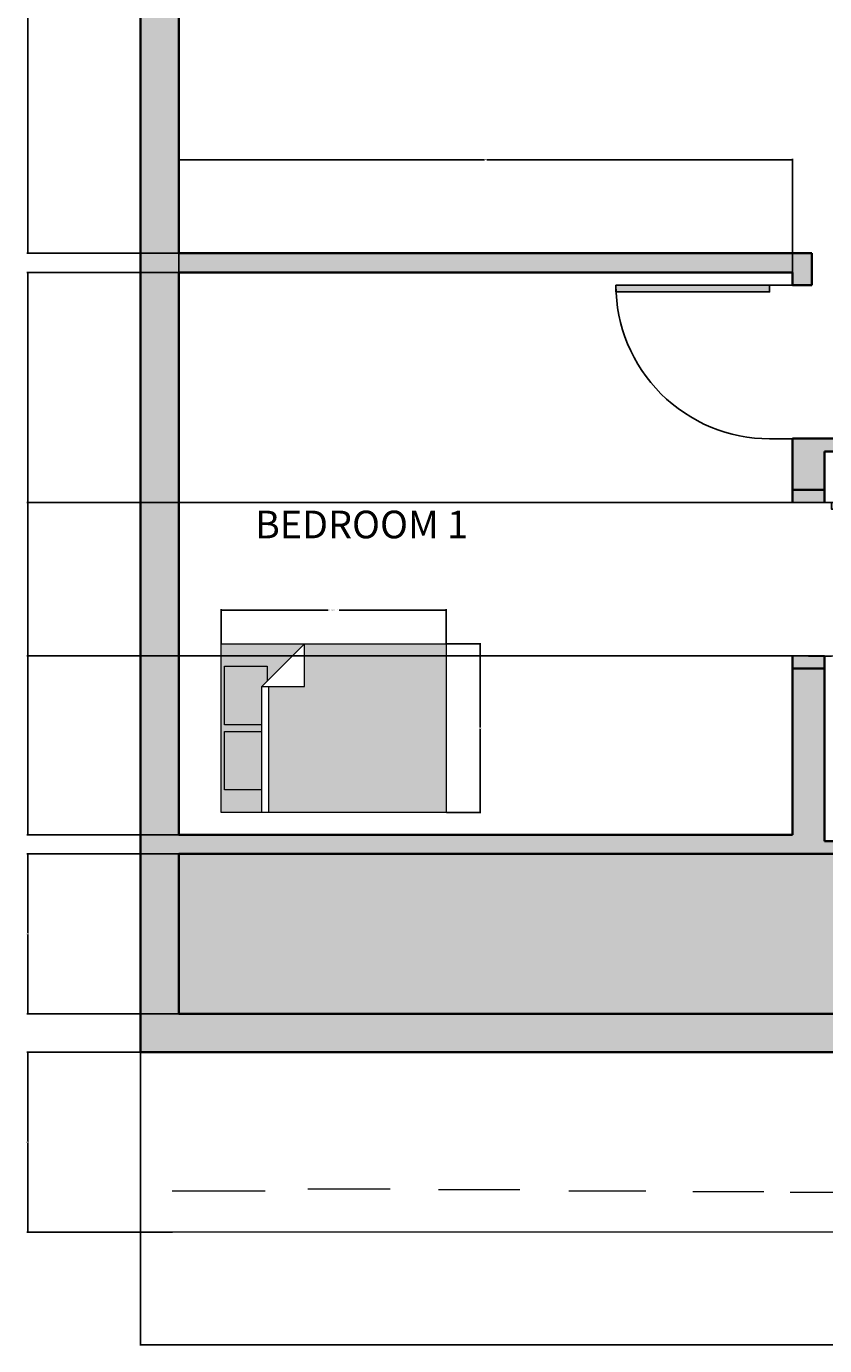
# Model space of a CAD drawing. Units: inches. Extents: x 1034 to 1730, y 674 to 1249.
# Tile 1 of 4: x 1316 to 1503, y 674 to 983. Entities that reach past the tile are written whole.
import ezdxf

# ---------------------------------------------------------------- set-up
doc = ezdxf.new("R2010")
doc.units = ezdxf.units.IN
for name, color, linetype, lineweight in [('A-ANNO-DIMS', 2, 'Continuous', 18), ('A-AREA-IDEN', 7, 'Continuous', 18), ('A-DOOR', 4, 'Continuous', 25), ('A-FURN', 9, 'Continuous', 18), ('A-FURN-PATT', 7, 'Continuous', 13), ('A-WALL', 7, 'Continuous', 35), ('A-WALL-PATT', 8, 'Continuous', 13), ('C-ROAD', 7, 'Continuous', 18)]:
    doc.layers.add(name, color=color, linetype=linetype, lineweight=lineweight)
doc.layers.add('A-DOOR-PATT', color=17, linetype='Continuous', lineweight=13, true_color=0x7b4636)
doc.layers.add('C-SITE-PATT', color=18, linetype='Continuous', lineweight=13, true_color=0x000000)
doc.styles.get("Standard").update_dxf_attribs({"font": 'arial.ttf'})
doc.dimstyles.get("Standard").update_dxf_attribs({"dimtxt": 0.18, "dimasz": 0.18, "dimexe": 0.18, "dimexo": 0.0625, "dimgap": 0.09, "dimtad": 0, "dimtih": 1, "dimtoh": 1, "dimdec": 4, "dimzin": 0, "dimdsep": 46, "dimtxsty": 'Standard', "dimcen": 0.09, "dimadec": 0, "dimazin": 0, "dimtfac": 1, "dimtdec": 4, "dimtofl": 0, "dimtmove": 0, "dimatfit": 3, "dimfxl": 1, "dimtolj": 1, "dimtzin": 0, "dimarcsym": 0})

# ---------------------------------------------------------------- blocks, each defined once
blk = doc.blocks.new('*U2')
for p, q in [((0, 0), (0, 6)), ((40, 0), (40, 6))]:
    blk.add_line(p, q)
blk.add_lwpolyline([(0, 0), (0, -40), (1.75, -40), (1.75, 0)], close=True)
blk.add_arc((0, 0), 40, 270, 0)
blk = doc.blocks.new('*U3')
for p, q in [((0, 0), (0, -6)), ((40, 0), (40, -6))]:
    blk.add_line(p, q)
blk.add_lwpolyline([(0, 0), (0, 40), (1.75, 40), (1.75, 0)], close=True)
blk.add_arc((0, 0), 40, 0, 90)
blk = doc.blocks.new('Bed - Queen')
for p, q in [((0, -80.00003), (0, 0)), ((0, 0), (59.99999, 0)), ((59.99999, 0), (59.99999, -80.00003)), ((7.99999, -1.2), (28.79998, -1.2)), ((7.99999, -14.4), (7.99999, -1.2)), ((28.79998, -1.2), (28.79998, -14.4)), ((31.19999, -1.2), (51.99999, -1.2)), ((31.19999, -14.4), (31.19999, -1.2)), ((51.99999, -1.2), (51.99999, -16.4)), ((0, -14.4), (44.8, -14.4)), ((44.8, -16.8), (0, -16.8)), ((59.99999, -29.6), (44.8, -14.4)), ((44.8, -14.4), (44.8, -29.6)), ((51.99999, -16.4), (46.79936, -16.4)), ((44.8, -29.6), (59.99999, -29.6)), ((59.99999, -80.00003), (0, -80.00003))]:
    blk.add_line(p, q)
blk = doc.blocks.new('*D8')
at = {"layer": 'A-ANNO-DIMS', "color": 0, "lineweight": -2, "transparency": 16777216}
for p, q in [((1361.47, 838.34), (1361.47, 846.37)), ((1361.65, 846.19), (1386.57, 846.19)), ((1414.1, 846.19), (1389.18, 846.19)), ((1414.28, 838.34), (1414.28, 846.37))]:
    blk.add_line(p, q, dxfattribs=at)
at = {"layer": 'A-ANNO-DIMS', "color": 0, "transparency": 16777216}
for points in [[(1361.65, 846.22), (1361.65, 846.16), (1361.47, 846.19)], [(1414.1, 846.22), (1414.1, 846.16), (1414.28, 846.19)]]:
    blk.add_solid(points, dxfattribs=at)
at = {"layer": 'Defpoints', "color": 0, "transparency": 16777216}
for p in [(1361.47, 846.19), (1361.47, 838.27), (1414.28, 838.27)]:
    blk.add_point(p, dxfattribs=at)
at = {"layer": 'A-ANNO-DIMS', "color": 0, "transparency": 16777216, "insert": (1387.87, 846.19), "char_height": 0.18, "attachment_point": 5}
blk.add_mtext('\\A1;QUEEN BED 53 TYP.', dxfattribs=at)
blk = doc.blocks.new('*D9')
at = {"layer": 'A-ANNO-DIMS', "color": 0, "lineweight": -2, "transparency": 16777216}
for p, q in [((1414.34, 838.27), (1422.38, 838.27)), ((1422.2, 838.09), (1422.2, 818.65)), ((1422.2, 798.85), (1422.2, 818.29)), ((1414.34, 798.67), (1422.38, 798.67))]:
    blk.add_line(p, q, dxfattribs=at)
at = {"layer": 'A-ANNO-DIMS', "color": 0, "transparency": 16777216}
for points in [[(1422.17, 838.09), (1422.23, 838.09), (1422.2, 838.27)], [(1422.17, 798.85), (1422.23, 798.85), (1422.2, 798.67)]]:
    blk.add_solid(points, dxfattribs=at)
at = {"layer": 'Defpoints', "color": 0, "transparency": 16777216}
for p in [(1414.28, 838.27), (1422.2, 838.27), (1414.28, 798.67)]:
    blk.add_point(p, dxfattribs=at)
at = {"layer": 'A-ANNO-DIMS', "color": 0, "transparency": 16777216, "insert": (1422.2, 818.47), "char_height": 0.18, "attachment_point": 5}
blk.add_mtext('\\A1;40 TYP.', dxfattribs=at)
blk = doc.blocks.new('*D14')
at = {"layer": 'A-ANNO-DIMS', "color": 0, "lineweight": -2, "transparency": 16777216}
for p, q in [((1342.53, 742.36), (1342.53, 673.53)), ((1702.53, 742.36), (1702.53, 673.53)), ((1342.71, 673.71), (1522.24, 673.71)), ((1702.35, 673.71), (1522.82, 673.71))]:
    blk.add_line(p, q, dxfattribs=at)
at = {"layer": 'A-ANNO-DIMS', "color": 0, "transparency": 16777216}
for points in [[(1342.71, 673.74), (1342.71, 673.68), (1342.53, 673.71)], [(1702.35, 673.74), (1702.35, 673.68), (1702.53, 673.71)]]:
    blk.add_solid(points, dxfattribs=at)
at = {"layer": 'Defpoints', "color": 0, "transparency": 16777216}
for p in [(1342.53, 742.43), (1702.53, 742.43), (1702.53, 673.71)]:
    blk.add_point(p, dxfattribs=at)
at = {"layer": 'A-ANNO-DIMS', "color": 0, "transparency": 16777216, "insert": (1522.53, 673.71), "char_height": 0.18, "attachment_point": 5}
blk.add_mtext('\\A1;360', dxfattribs=at)
blk = doc.blocks.new('*D16')
at = {"layer": 'A-ANNO-DIMS', "color": 0, "lineweight": -2, "transparency": 16777216}
for p, q in [((1342.47, 742.43), (1315.9, 742.43)), ((1316.08, 742.25), (1316.08, 721.48)), ((1316.08, 700.34), (1316.08, 721.11)), ((1350.03, 700.16), (1315.9, 700.16))]:
    blk.add_line(p, q, dxfattribs=at)
at = {"layer": 'A-ANNO-DIMS', "color": 0, "transparency": 16777216}
for points in [[(1316.05, 742.25), (1316.11, 742.25), (1316.08, 742.43)], [(1316.05, 700.34), (1316.11, 700.34), (1316.08, 700.16)]]:
    blk.add_solid(points, dxfattribs=at)
at = {"layer": 'Defpoints', "color": 0, "transparency": 16777216}
for p in [(1342.53, 742.43), (1316.08, 700.16), (1350.1, 700.16)]:
    blk.add_point(p, dxfattribs=at)
at = {"layer": 'A-ANNO-DIMS', "color": 0, "transparency": 16777216, "insert": (1316.08, 721.29), "char_height": 0.18, "attachment_point": 5}
blk.add_mtext('\\A1;42.26', dxfattribs=at)
blk = doc.blocks.new('*D20')
at = {"layer": 'A-ANNO-DIMS', "color": 0, "lineweight": -2, "transparency": 16777216}
for p, q in [((1351.47, 1088.93), (1315.9, 1088.93)), ((1316.08, 1088.75), (1316.08, 1009.61)), ((1316.08, 930.11), (1316.08, 1009.24)), ((1351.47, 929.93), (1315.9, 929.93))]:
    blk.add_line(p, q, dxfattribs=at)
at = {"layer": 'A-ANNO-DIMS', "color": 0, "transparency": 16777216}
for points in [[(1316.05, 1088.75), (1316.11, 1088.75), (1316.08, 1088.93)], [(1316.05, 930.11), (1316.11, 930.11), (1316.08, 929.93)]]:
    blk.add_solid(points, dxfattribs=at)
at = {"layer": 'Defpoints', "color": 0, "transparency": 16777216}
for p in [(1316.08, 1088.93), (1351.53, 1088.93), (1351.53, 929.93)]:
    blk.add_point(p, dxfattribs=at)
at = {"layer": 'A-ANNO-DIMS', "color": 0, "transparency": 16777216, "insert": (1316.08, 1009.43), "char_height": 0.18, "attachment_point": 5}
blk.add_mtext('\\A1;159', dxfattribs=at)
blk = doc.blocks.new('*D21')
at = {"layer": 'A-ANNO-DIMS', "color": 0, "lineweight": -2, "transparency": 16777216}
for p, q in [((1351.47, 925.43), (1315.9, 925.43)), ((1316.08, 925.25), (1316.08, 859.61)), ((1316.08, 793.61), (1316.08, 859.24)), ((1351.47, 793.43), (1315.9, 793.43))]:
    blk.add_line(p, q, dxfattribs=at)
at = {"layer": 'A-ANNO-DIMS', "color": 0, "transparency": 16777216}
for points in [[(1316.05, 925.25), (1316.11, 925.25), (1316.08, 925.43)], [(1316.05, 793.61), (1316.11, 793.61), (1316.08, 793.43)]]:
    blk.add_solid(points, dxfattribs=at)
at = {"layer": 'Defpoints', "color": 0, "transparency": 16777216}
for p in [(1316.08, 925.43), (1351.53, 925.43), (1351.53, 793.43)]:
    blk.add_point(p, dxfattribs=at)
at = {"layer": 'A-ANNO-DIMS', "color": 0, "transparency": 16777216, "insert": (1316.08, 859.43), "char_height": 0.18, "attachment_point": 5}
blk.add_mtext('\\A1;132', dxfattribs=at)
blk = doc.blocks.new('*D22')
at = {"layer": 'A-ANNO-DIMS', "color": 0, "lineweight": -2, "transparency": 16777216}
for p, q in [((1351.47, 788.93), (1315.9, 788.93)), ((1316.08, 788.75), (1316.08, 770.36)), ((1316.08, 751.61), (1316.08, 769.99)), ((1351.47, 751.43), (1315.9, 751.43))]:
    blk.add_line(p, q, dxfattribs=at)
at = {"layer": 'A-ANNO-DIMS', "color": 0, "transparency": 16777216}
for points in [[(1316.05, 788.75), (1316.11, 788.75), (1316.08, 788.93)], [(1316.05, 751.61), (1316.11, 751.61), (1316.08, 751.43)]]:
    blk.add_solid(points, dxfattribs=at)
at = {"layer": 'Defpoints', "color": 0, "transparency": 16777216}
for p in [(1316.08, 788.93), (1351.53, 788.93), (1351.53, 751.43)]:
    blk.add_point(p, dxfattribs=at)
at = {"layer": 'A-ANNO-DIMS', "color": 0, "transparency": 16777216, "insert": (1316.08, 770.18), "char_height": 0.18, "attachment_point": 5}
blk.add_mtext('\\A1;37.5', dxfattribs=at)
blk = doc.blocks.new('*D23')
at = {"layer": 'A-ANNO-DIMS', "color": 0, "lineweight": -2, "transparency": 16777216}
for p, q in [((1351.53, 925.49), (1351.53, 952.06)), ((1351.71, 951.88), (1423.25, 951.88)), ((1495.35, 951.88), (1423.81, 951.88)), ((1495.53, 925.49), (1495.53, 952.06))]:
    blk.add_line(p, q, dxfattribs=at)
at = {"layer": 'A-ANNO-DIMS', "color": 0, "transparency": 16777216}
for points in [[(1351.71, 951.91), (1351.71, 951.85), (1351.53, 951.88)], [(1495.35, 951.91), (1495.35, 951.85), (1495.53, 951.88)]]:
    blk.add_solid(points, dxfattribs=at)
at = {"layer": 'Defpoints', "color": 0, "transparency": 16777216}
for p in [(1495.53, 951.88), (1351.53, 925.43), (1495.53, 925.43)]:
    blk.add_point(p, dxfattribs=at)
at = {"layer": 'A-ANNO-DIMS', "color": 0, "transparency": 16777216, "insert": (1423.53, 951.88), "char_height": 0.18, "attachment_point": 5}
blk.add_mtext('\\A1;144', dxfattribs=at)
blk = doc.blocks.new('*D31')
at = {"layer": 'A-ANNO-DIMS', "color": 0, "lineweight": -2, "transparency": 16777216}
for p, q in [((1495.47, 871.43), (1315.9, 871.43)), ((1316.08, 871.25), (1316.08, 853.61)), ((1316.08, 835.61), (1316.08, 853.24)), ((1495.47, 835.43), (1315.9, 835.43))]:
    blk.add_line(p, q, dxfattribs=at)
at = {"layer": 'A-ANNO-DIMS', "color": 0, "transparency": 16777216}
for points in [[(1316.05, 871.25), (1316.11, 871.25), (1316.08, 871.43)], [(1316.05, 835.61), (1316.11, 835.61), (1316.08, 835.43)]]:
    blk.add_solid(points, dxfattribs=at)
at = {"layer": 'Defpoints', "color": 0, "transparency": 16777216}
for p in [(1316.08, 871.43), (1495.53, 871.43), (1495.53, 835.43)]:
    blk.add_point(p, dxfattribs=at)
at = {"layer": 'A-ANNO-DIMS', "color": 0, "transparency": 16777216, "insert": (1316.08, 853.43), "char_height": 0.18, "attachment_point": 5}
blk.add_mtext('\\A1;36', dxfattribs=at)
blk = doc.blocks.new('*D32')
at = {"layer": 'A-ANNO-DIMS', "color": 0, "lineweight": -2, "transparency": 16777216}
for p, q in [((1495.47, 835.43), (1315.9, 835.43)), ((1316.08, 835.25), (1316.08, 814.61)), ((1316.08, 793.61), (1316.08, 814.25)), ((1495.47, 793.43), (1315.9, 793.43))]:
    blk.add_line(p, q, dxfattribs=at)
at = {"layer": 'A-ANNO-DIMS', "color": 0, "transparency": 16777216}
for points in [[(1316.05, 835.25), (1316.11, 835.25), (1316.08, 835.43)], [(1316.05, 793.61), (1316.11, 793.61), (1316.08, 793.43)]]:
    blk.add_solid(points, dxfattribs=at)
at = {"layer": 'Defpoints', "color": 0, "transparency": 16777216}
for p in [(1495.53, 835.43), (1316.08, 793.43), (1495.53, 793.43)]:
    blk.add_point(p, dxfattribs=at)
at = {"layer": 'A-ANNO-DIMS', "color": 0, "transparency": 16777216, "insert": (1316.08, 814.43), "char_height": 0.18, "attachment_point": 5}
blk.add_mtext('\\A1;42', dxfattribs=at)

msp = doc.modelspace()

# ---------------------------------------------------------------- hatches: boundary and pattern name
at = {"layer": 'A-DOOR-PATT'}
h = msp.add_hatch(color=256, dxfattribs=at)
h.dxf.hatch_style = 1
h.paths.add_polyline_path([(1490.123, 922.4262), (1454.0839, 922.4262, 0.01094143), (1454.1184, 920.8495), (1490.123, 920.8495)])
h.paths.add_polyline_path([(1540.7238, 871.4262), (1504.6847, 871.4262), (1504.6847, 869.8495), (1540.6893, 869.8495, 0.01094143)])
h.paths.add_polyline_path([(1503.0288, 874.4262), (1495.5288, 874.4262), (1495.5288, 871.4262), (1503.0288, 871.4262)])
h.paths.add_polyline_path([(1503.0288, 835.3871), (1499.2788, 835.3871), (1495.5288, 835.4262), (1495.5288, 832.4262), (1503.0288, 832.4262)])
h.paths.add_polyline_path([(1564.6056, 873.3367, 0.01094143), (1563.0288, 873.3712), (1563.0288, 837.3321), (1564.6056, 837.3321)])
h.paths.add_polyline_path([(1602.0288, 831.9262), (1599.0288, 831.9262), (1599.0288, 828.9262), (1602.0288, 828.9262)])
h.paths.add_polyline_path([(1648.5288, 988.4262), (1645.5288, 988.4262), (1645.5288, 985.4262), (1648.5288, 985.4262)])
h.paths.add_polyline_path([(1689.9738, 989.9638), (1653.9347, 989.9638), (1653.9347, 988.3871), (1689.9738, 988.3871)])
h.paths.add_polyline_path([(1648.5288, 1027.4262), (1645.5288, 1027.4262), (1645.5288, 1024.4262), (1648.5288, 1024.4262)])
h.paths.add_polyline_path([(1590.9393, 1097.9638), (1554.9347, 1097.9638), (1554.9347, 1096.3871), (1590.9738, 1096.3871, 0.01094143)])
h.paths.add_polyline_path([(1549.5288, 1135.4262), (1545.0288, 1135.4262), (1545.0288, 1132.4262), (1549.5288, 1132.4262)])
h.paths.add_polyline_path([(1500.0288, 1135.4262), (1495.5288, 1135.4262), (1495.5288, 1132.4262), (1500.0288, 1132.4262)])
h.paths.add_polyline_path([(1490.123, 1098.0029), (1454.0839, 1098.0029), (1454.0839, 1096.4262), (1490.123, 1096.4262)])
h.paths.add_polyline_path([(1539.068, 1194.8712, 0.01094143), (1537.4912, 1194.8367), (1537.4912, 1158.8321), (1539.068, 1158.8321)])
at = {"layer": 'A-FURN-PATT'}
h = msp.add_hatch(color=256, dxfattribs=at)
h.dxf.hatch_style = 1
h.paths.add_polyline_path([(1414.278, 838.2731), (1381.0078, 838.2731), (1381.0078, 828.2392), (1372.5582, 828.2392), (1372.5582, 798.6657), (1414.278, 798.6657)])
h.paths.add_polyline_path([(1370.9739, 828.2392), (1372.2941, 829.5594), (1372.2941, 832.9921), (1362.2603, 832.9921), (1362.2603, 819.2615), (1370.9739, 819.2615)], flags=17)
h.paths.add_polyline_path([(1370.9739, 817.6772), (1362.2603, 817.6772), (1362.2603, 803.9467), (1370.9739, 803.9467)], flags=17)
h.paths.add_polyline_path([(1367.0568, 1198.6055), (1368.377, 1199.9257), (1368.377, 1203.3584), (1358.3431, 1203.3584), (1358.3431, 1189.6278), (1367.0568, 1189.6278)], flags=17)
h.paths.add_polyline_path([(1367.0568, 1188.0435), (1358.3431, 1188.0435), (1358.3431, 1174.3129), (1367.0568, 1174.3129)], flags=17)
h.paths.add_polyline_path([(1410.3609, 1208.6394), (1377.0906, 1208.6394), (1377.0906, 1198.6055), (1368.6411, 1198.6055), (1368.6411, 1169.032), (1410.3609, 1169.032)])
h.paths.add_polyline_path([(1678.2824, 1203.4604), (1636.5626, 1203.4604), (1636.5626, 1163.853), (1669.8329, 1163.853), (1669.8329, 1173.8868), (1678.2824, 1173.8868)])
h.paths.add_polyline_path([(1688.5804, 1182.8645), (1679.8667, 1182.8645), (1679.8667, 1173.8868), (1678.5465, 1172.5666), (1678.5465, 1169.1339), (1688.5804, 1169.1339)], flags=17)
h.paths.add_polyline_path([(1367.0568, 1174.3129), (1358.3431, 1174.3129), (1358.3431, 1188.0435), (1367.0568, 1188.0435), (1367.0568, 1189.6278), (1358.3431, 1189.6278), (1358.3431, 1203.3584), (1368.377, 1203.3584), (1368.377, 1199.9257), (1377.0906, 1208.6394), (1357.551, 1208.6394), (1357.551, 1169.032), (1367.0568, 1169.032)])
h.paths.add_polyline_path([(1688.5804, 1198.1794), (1679.8667, 1198.1794), (1679.8667, 1184.4488), (1688.5804, 1184.4488)], flags=17)
h.paths.add_polyline_path([(1689.3725, 1203.4604), (1679.8667, 1203.4604), (1679.8667, 1198.1794), (1688.5804, 1198.1794), (1688.5804, 1184.4488), (1679.8667, 1184.4488), (1679.8667, 1182.8645), (1688.5804, 1182.8645), (1688.5804, 1169.1339), (1678.5465, 1169.1339), (1678.5465, 1172.5666), (1669.8329, 1163.853), (1689.3725, 1163.853)])
h.paths.add_polyline_path([(1370.9739, 803.9467), (1362.2603, 803.9467), (1362.2603, 817.6772), (1370.9739, 817.6772), (1370.9739, 819.2615), (1362.2603, 819.2615), (1362.2603, 832.9921), (1372.2941, 832.9921), (1372.2941, 829.5594), (1381.0078, 838.2731), (1361.4681, 838.2731), (1361.4681, 798.6657), (1370.9739, 798.6657)])
h.paths.add_polyline_path([(1586.4252, 1162.5974), (1646.7165, 1162.5974), (1646.7165, 1172.6784), (1586.4252, 1172.6784)], flags=9)
h.paths.add_polyline_path([(1574.2942, 863.9077), (1611.4062, 863.9077), (1611.4062, 873.9821), (1574.2942, 873.9821)], flags=9)
h.paths.add_polyline_path([(1502.8652, 818.6383), (1550.5629, 818.6383), (1550.5629, 828.7127), (1502.8652, 828.7127)], flags=9)
h.paths.add_polyline_path([(1367.7365, 861.2327), (1425.5064, 861.2327), (1425.5064, 871.3071), (1367.7365, 871.3071)], flags=9)
h.paths.add_polyline_path([(1409.7909, 1010.2859), (1487.2071, 1010.2859), (1487.2071, 1020.3537), (1409.7909, 1020.3537)], flags=9)
h.paths.add_polyline_path([(1499.9637, 1199.6865), (1545.1423, 1199.6865), (1545.1423, 1209.7608), (1499.9637, 1209.7608)], flags=9)
h.paths.add_polyline_path([(1378.5639, 1158.2313), (1436.3338, 1158.2313), (1436.3338, 1168.3057), (1378.5639, 1168.3057)], flags=9)
at = {"layer": 'A-WALL-PATT'}
h = msp.add_hatch(color=256, dxfattribs=at)
h.dxf.hatch_style = 1
h.paths.add_polyline_path([(1351.5288, 1213.4262), (1495.5288, 1213.4262), (1495.5288, 1135.4262), (1500.0288, 1135.4262), (1500.0288, 1148.9262), (1503.0288, 1148.9262), (1503.0288, 1153.4262), (1500.0288, 1153.4262), (1500.0288, 1213.4262), (1545.0288, 1213.4262), (1545.0288, 1153.4262), (1539.0288, 1153.4262), (1539.0288, 1148.9262), (1545.0288, 1148.9262), (1545.0288, 1135.4262), (1549.5288, 1135.4262), (1549.5288, 1213.4262), (1693.5288, 1213.4262), (1693.5288, 1093.4262), (1549.5288, 1093.4262), (1549.5288, 1096.4262), (1545.0288, 1096.4262), (1545.0288, 1088.9262), (1549.5288, 1088.9262), (1549.5288, 1064.9262), (1552.5288, 1064.9262), (1552.5288, 1088.9262), (1645.5288, 1088.9262), (1645.5288, 1027.4262), (1648.5288, 1027.4262), (1648.5288, 1088.9262), (1693.5288, 1088.9262), (1693.5288, 985.4262), (1552.5288, 985.4262), (1552.5288, 1004.9262), (1549.5288, 1004.9262), (1549.5288, 980.9262), (1620.0288, 980.9262), (1620.0288, 831.9262), (1602.0288, 831.9262), (1602.0288, 828.9262), (1624.5288, 828.9262), (1624.5288, 980.9262), (1693.5288, 980.9262), (1693.5288, 742.4262), (1702.5288, 742.4262), (1702.5288, 1222.4262), (1342.5288, 1222.4262), (1342.5288, 742.4262), (1620.0288, 742.4262), (1620.0288, 751.4262), (1351.5288, 751.4262), (1351.5288, 788.9262), (1560.0288, 788.9262), (1560.0288, 828.9262), (1563.0288, 828.9262), (1563.0288, 831.9262), (1560.0288, 831.9262), (1560.0288, 886.4262), (1500.0288, 886.4262), (1495.5288, 886.4262), (1495.5288, 874.4262), (1503.0288, 874.4262), (1503.0288, 883.4262), (1557.0288, 883.4262), (1557.0288, 791.9262), (1503.0288, 791.9262), (1503.0288, 832.4262), (1495.5288, 832.4262), (1495.5288, 793.4262), (1351.5288, 793.4262), (1351.5288, 925.4262), (1495.5288, 925.4262), (1495.5288, 922.4262), (1500.0288, 922.4262), (1500.0288, 929.9262), (1351.5288, 929.9262), (1351.5288, 1088.9262), (1500.0288, 1088.9262), (1500.0288, 1096.4262), (1495.5288, 1096.4262), (1495.5288, 1093.4262), (1351.5288, 1093.4262)])
at = {"layer": 'C-SITE-PATT'}
h = msp.add_hatch(color=256, dxfattribs=at)
h.dxf.hatch_style = 1
h.paths.add_polyline_path([(1620.0288, 778.9262), (1560.0288, 778.9262), (1560.0288, 788.9262), (1351.5288, 788.9262), (1351.5288, 751.4262), (1620.0288, 751.4262)])

# ---------------------------------------------------------------- linework, layer by layer
at = {"layer": 'A-DOOR'}
for p, q in [((1495.5288, 871.4262), (1503.0288, 871.4262)), ((1495.5288, 835.4262), (1503.0288, 835.4262))]:
    msp.add_line(p, q, dxfattribs=at)
at = {"layer": 'A-WALL'}
for p, q in [((1351.5288, 929.9262), (1351.5288, 1088.9262)), ((1351.5288, 929.9262), (1500.0288, 929.9262)), ((1500.0288, 922.4262), (1500.0288, 929.9262)), ((1351.5288, 925.4262), (1495.5288, 925.4262)), ((1351.5288, 793.4262), (1351.5288, 925.4262)), ((1495.5288, 922.4262), (1495.5288, 925.4262)), ((1495.5288, 922.4262), (1500.0288, 922.4262)), ((1495.5288, 886.4262), (1500.0288, 886.4262)), ((1495.5288, 871.4262), (1495.5288, 886.4262)), ((1560.0288, 886.4262), (1500.0288, 886.4262)), ((1557.0288, 883.4262), (1503.0288, 883.4262)), ((1503.0288, 871.4262), (1503.0288, 883.4262)), ((1495.5288, 874.4262), (1503.0288, 874.4262)), ((1495.5288, 793.4262), (1495.5288, 835.4262)), ((1503.0288, 791.9262), (1503.0288, 835.4262)), ((1495.5288, 832.4262), (1503.0288, 832.4262)), ((1351.5288, 793.4262), (1495.5288, 793.4262)), ((1503.0288, 791.9262), (1557.0288, 791.9262)), ((1351.5288, 751.4262), (1351.5288, 788.9262)), ((1351.5288, 788.9262), (1560.0288, 788.9262)), ((1620.0288, 751.4262), (1351.5288, 751.4262))]:
    msp.add_line(p, q, dxfattribs=at)
msp.add_lwpolyline([(1620.0288, 742.4262), (1342.5288, 742.4262), (1342.5288, 1222.4262), (1702.5288, 1222.4262), (1702.5288, 742.4262), (1693.5288, 742.4262)], dxfattribs=at)
at = {"layer": 'C-ROAD'}
for p, q in [((1349.9974, 709.8276), (1371.7731, 709.8276)), ((1381.8314, 710.3456), (1401.1184, 710.3456)), ((1412.4211, 710.1384), (1431.5007, 710.1384)), ((1443.0484, 709.829), (1461.0911, 709.829)), ((1472.0944, 709.7248), (1488.7891, 709.7248)), ((1494.9352, 709.5884), (1511.7588, 709.5884)), ((1703.0641, 700.1632), (1350.0973, 700.1632))]:
    msp.add_line(p, q, dxfattribs=at)

# ---------------------------------------------------------------- block references
at = {"layer": 'A-DOOR', "xscale": 0.9009776753840846, "yscale": 0.9009776753840846, "zscale": 0.9009776753840846, "rotation": 270}
for name, p in [('*U2', (1490.123, 922.4262)), ('*U3', (1504.6847, 871.4262))]:
    msp.add_blockref(name, p, dxfattribs=at)
at = {"layer": 'A-FURN', "xscale": 0.6601233642522663, "yscale": 0.6601233642522663, "zscale": 0.6601233642522663, "rotation": 90}
msp.add_blockref('Bed - Queen', (1361.4681, 798.6657), dxfattribs=at)

# ---------------------------------------------------------------- texts
at = {"layer": 'A-AREA-IDEN'}
msp.add_text('BEDROOM 1', height=6.49045, dxfattribs=at).set_placement((1369.4156, 863.0225))

# ---------------------------------------------------------------- dimensions: what is measured, and where the dimension line sits
at = {"layer": 'A-ANNO-DIMS'}
for base, p1, p2, override, picture, middle in [((1316.0788, 1088.9262), (1351.5288, 929.9262), (1351.5288, 1088.9262), {"dimdec": 0, "dimlfac": 1, "dimrnd": 0, "dimzin": 0, "dimdsep": 46, "dimlunit": 2}, '*D20', (1316.0788, 1009.4262)), ((1316.0788, 925.4262), (1351.5288, 793.4262), (1351.5288, 925.4262), {"dimdec": 0, "dimlfac": 1, "dimrnd": 0, "dimzin": 0, "dimdsep": 46, "dimlunit": 2}, '*D21', (1316.0788, 859.4262)), ((1316.0788, 871.4262), (1495.5288, 835.4262), (1495.5288, 871.4262), {"dimdec": 0, "dimlfac": 1, "dimrnd": 0, "dimzin": 0, "dimdsep": 46, "dimlunit": 2}, '*D31', (1316.0788, 853.4262)), ((1316.0788, 793.4262), (1495.5288, 835.4262), (1495.5288, 793.4262), {"dimdec": 0, "dimlfac": 1, "dimrnd": 0, "dimzin": 0, "dimdsep": 46, "dimlunit": 2}, '*D32', (1316.0788, 814.4262)), ((1316.0788, 788.9262), (1351.5288, 751.4262), (1351.5288, 788.9262), {"dimdec": 1, "dimlfac": 1, "dimrnd": 0, "dimzin": 0, "dimdsep": 46, "dimlunit": 2}, '*D22', (1316.0788, 770.1762)), ((1316.0788, 700.1632), (1342.5288, 742.4262), (1350.0973, 700.1632), {"dimdec": 2, "dimlfac": 1, "dimrnd": 0, "dimzin": 0, "dimdsep": 46, "dimlunit": 2}, '*D16', (1316.0788, 721.2947))]:
    dim = msp.add_linear_dim(base=base, p1=p1, p2=p2, angle=90, dimstyle='Standard', override=override, dxfattribs=at)
    dim.commit()
    dim.dimension.update_dxf_attribs({"geometry": picture, "text_midpoint": middle})
for base, p1, p2, picture, middle in [((1495.5288, 951.8762), (1351.5288, 925.4262), (1495.5288, 925.4262), '*D23', (1423.5288, 951.8762)), ((1702.5288, 673.7132), (1342.5288, 742.4262), (1702.5288, 742.4262), '*D14', (1522.5288, 673.7132))]:
    dim = msp.add_linear_dim(base=base, p1=p1, p2=p2, dimstyle='Standard', override={"dimdec": 0, "dimlfac": 1, "dimrnd": 0, "dimzin": 0, "dimdsep": 46, "dimlunit": 2}, dxfattribs=at)
    dim.commit()
    dim.dimension.update_dxf_attribs({"geometry": picture, "text_midpoint": middle})
for base, p1, p2, angle, text, picture, middle in [((1361.4681, 846.1946), (1414.278, 838.2731), (1361.4681, 838.2731), 180, 'QUEEN BED <> TYP.', '*D8', (1387.8731, 846.1946)), ((1422.1995, 838.2731), (1414.278, 798.6657), (1414.278, 838.2731), 90, '<> TYP.', '*D9', (1422.1995, 818.4694))]:
    dim = msp.add_linear_dim(base=base, p1=p1, p2=p2, angle=angle, text=text, dimstyle='Standard', override={"dimdec": 0, "dimlfac": 1, "dimrnd": 0, "dimzin": 0, "dimdsep": 46, "dimlunit": 2}, dxfattribs=at)
    dim.commit()
    dim.dimension.update_dxf_attribs({"geometry": picture, "text_midpoint": middle})

doc.saveas('drawing.dxf')
